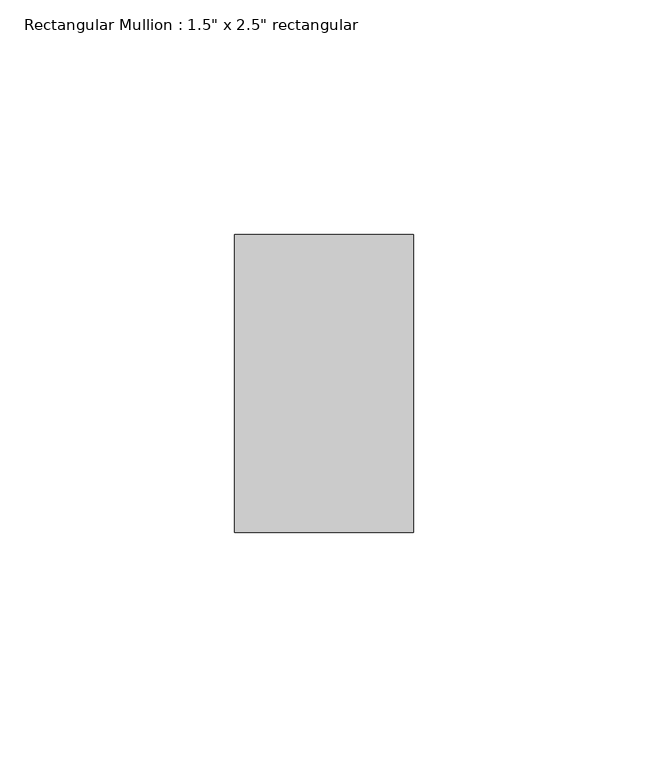
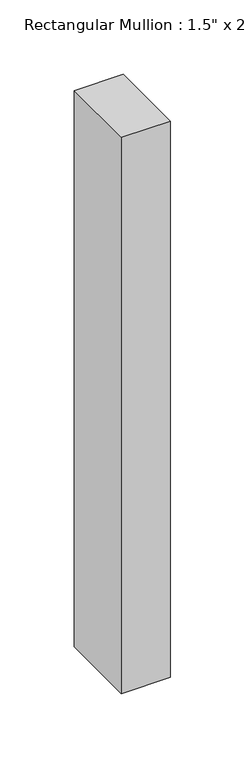
"""IFC4 building model written with IfcOpenShell, lengths in millimetres: member geometry."""

from ifc_helpers import new_model, si_unit, frame, origin, place, context, project, spatial, polyline, outline, extrude, source, transform, mapped, element, save


def member_bf4473fa(model_context):
    return source(origin(), model_context, "Body", "SweptSolid", [
        extrude(outline(polyline([(19.05, 31.75), (19.05, -31.75), (-19.05, -31.75), (-19.05, 31.75), (19.05, 31.75)])), frame((0.0, 0.0, -457.2), z_axis=(0.0, 0.0, 1.0), x_axis=(1.0, 0.0, 0.0)), (0.0, 0.0, 1.0), 457.2),
    ])


if __name__ == "__main__":
    model = new_model("IFC4")
    model_context = context("Model", 3, world=origin())
    ifc_project = project(units=[si_unit("LENGTHUNIT", "METRE", prefix="MILLI")], contexts=[model_context])
    site = spatial("IfcSite", under=ifc_project)
    building = spatial("IfcBuilding", under=site)
    placement = place(None, origin())
    member_shape = member_bf4473fa(model_context)
    element("IfcMember", 1, ObjectType="Rectangular Mullion : 1.5\" x 2.5\" rectangular", at=placement, inside=building, context=model_context, shape_type="MappedRepresentation", body=[
        mapped(member_shape, transform((0.0, 0.0, 0.0), x_axis=(1.0, 0.0, 0.0), y_axis=(0.0, 1.0, 0.0), z_axis=(0.0, 0.0, 1.0))),
    ])
    save(model, "model.ifc")

# Revit data of these elements
# Type "Rectangular Mullion : 1.5\" x 2.5\" rectangular"
#   built-in parameter 1007304 = 0.208333 (stored number, unit not read)
#   built-in parameter 1007301 = 0.0625 (stored number, unit not read)
#   built-in parameter 1007300 = 0.0625 (stored number, unit not read)
# Element 1 (IfcMember, "Rectangular Mullion : 1.5\" x 2.5\" rectangular")
#   Materials on its faces: "Leather - Black"
# Materials
#   "Leather - Black": class "Generic", colour RGB 40 40 40, transparency 0, Cost = 0
